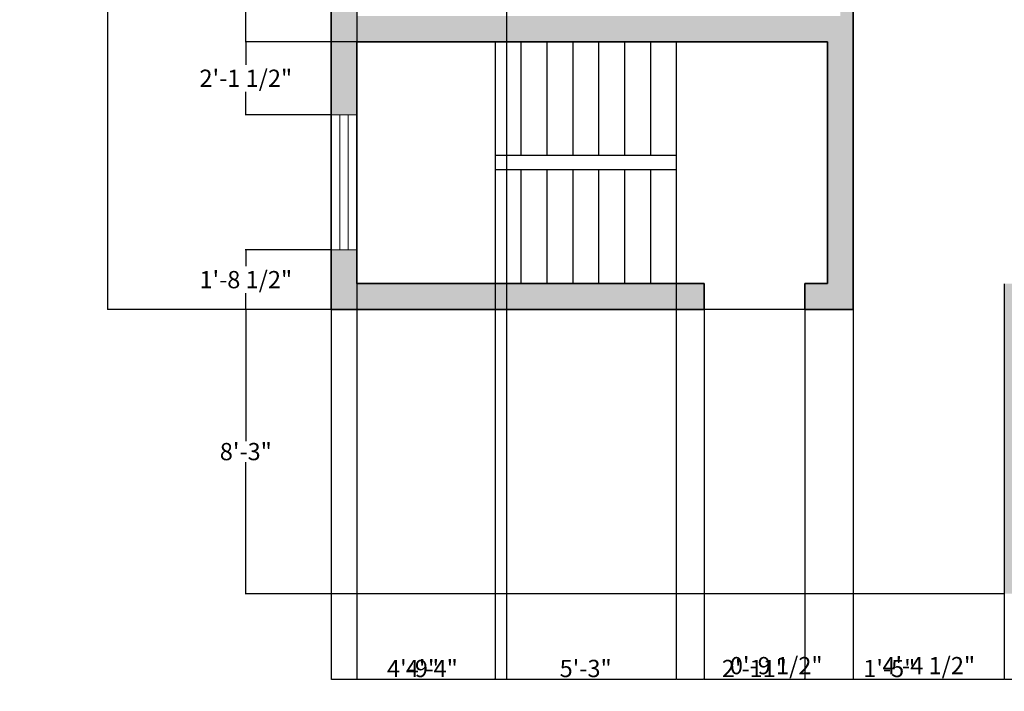
# Model space of a CAD drawing. Units: inches. Extents: x 2322 to 2932, y 142 to 762.
# Tile 1 of 7: x 2322 to 2664, y 142 to 376. Entities that reach past the tile are written whole.
import ezdxf

# ---------------------------------------------------------------- set-up
doc = ezdxf.new("R2010")
doc.units = ezdxf.units.IN
doc.header["$MEASUREMENT"] = 0
for name, color, linetype, lineweight in [('A-ANNO-DIMS', 2, 'Continuous', 18), ('A-FLOR-STRS', 7, 'Continuous', 25), ('A-GLAZ', 4, 'Continuous', 18), ('A-WALL', 7, 'Continuous', 35)]:
    doc.layers.add(name, color=color, linetype=linetype, lineweight=lineweight)
doc.layers.add('A-WALL-PATT', color=40, linetype='Continuous', lineweight=13, true_color=0xf8d731)
doc.styles.get("Standard").update_dxf_attribs({"font": 'italic8.shx'})
doc.dimstyles.get("Standard").update_dxf_attribs({"dimtxt": 6, "dimasz": 0.15, "dimexe": 0.18, "dimexo": 0.0625, "dimgap": 0.09, "dimtad": 1, "dimtih": 1, "dimtoh": 1, "dimzin": 0, "dimdsep": 46, "dimlunit": 3, "dimtxsty": 'Standard', "dimblk": 'CLOSEDBLANK', "dimcen": 0.09, "dimclrd": 3, "dimclre": 1, "dimclrt": 6, "dimadec": 0, "dimazin": 0, "dimtfac": 1, "dimtofl": 0, "dimtmove": 0, "dimatfit": 3, "dimldrblk": 'DOT', "dimfxl": 1, "dimtolj": 1, "dimtzin": 0, "dimarcsym": 0})

# ---------------------------------------------------------------- blocks, each defined once
blk = doc.blocks.new('_ClosedBlank')
at = {"color": 0, "linetype": 'ByBlock', "lineweight": -2}
for p, q in [((-1, 0.2), (0, 0)), ((-1, 0.2), (-1, -0.2)), ((0, 0), (-1, -0.2))]:
    blk.add_line(p, q, dxfattribs=at)
blk = doc.blocks.new('*D8')
at = {"layer": 'A-ANNO-DIMS', "color": 0, "lineweight": -2, "transparency": 16777216}
for p, q in [((2430, 718.82), (2352.33, 718.82)), ((2352.51, 718.67), (2352.51, 501.45)), ((2352.51, 274.91), (2352.51, 492.13)), ((2430, 274.76), (2352.33, 274.76))]:
    blk.add_line(p, q, dxfattribs=at)
at = {"layer": 'Defpoints', "color": 0, "transparency": 16777216}
for p in [(2430.06, 718.82), (2352.51, 274.76), (2430.06, 274.76)]:
    blk.add_point(p, dxfattribs=at)
at = {"layer": 'A-ANNO-DIMS', "color": 0, "lineweight": -2, "transparency": 16777216, "xscale": 0.15, "yscale": 0.15, "zscale": 0.15}
for p, rotation in [((2352.51, 718.82), 90), ((2352.51, 274.76), 270)]:
    blk.add_blockref('_ClosedBlank', p, dxfattribs=dict(at, rotation=rotation))
at = {"layer": 'A-ANNO-DIMS', "color": 0, "transparency": 16777216, "insert": (2352.51, 496.79), "char_height": 6, "attachment_point": 5}
blk.add_mtext('\\A1;37\'-0.06" [11.28]', dxfattribs=at)
blk = doc.blocks.new('_Dot')
at = {"color": 0, "linetype": 'ByBlock', "lineweight": -2}
blk.add_line((-0.5, 0), (-1, 0), dxfattribs=at)
at = {"color": 0, "linetype": 'ByBlock', "const_width": 0.5}
blk.add_lwpolyline([(-0.25, 0, 1), (0.25, 0, 1)], format="xyb", close=True, dxfattribs=at)
blk = doc.blocks.new('WINDOW-47X9')
for p, q in [((47, 9), (0, 9)), ((0, 9), (0, 0)), ((47, 0), (47, 9)), ((0, 6), (47, 6)), ((0, 3), (47, 3)), ((0, 0), (47, 0))]:
    blk.add_line(p, q)
blk = doc.blocks.new('*D44')
at = {"layer": 'A-ANNO-DIMS', "color": 1, "lineweight": -2, "transparency": 16777216}
for p, q in [((2487.06, 283.69), (2487.06, 146.01)), ((2430.06, 274.69), (2430.06, 146.01))]:
    blk.add_line(p, q, dxfattribs=at)
at = {"layer": 'A-ANNO-DIMS', "color": 3, "lineweight": -2, "transparency": 16777216}
blk.add_line((2430.21, 146.19), (2486.91, 146.19), dxfattribs=at)
at = {"layer": 'Defpoints', "color": 0, "transparency": 16777216}
for p in [(2487.06, 283.76), (2430.06, 274.76), (2487.06, 146.19)]:
    blk.add_point(p, dxfattribs=at)
at = {"layer": 'A-ANNO-DIMS', "color": 3, "lineweight": -2, "transparency": 16777216, "xscale": 0.15, "yscale": 0.15, "zscale": 0.15, "rotation": 180}
blk.add_blockref('_ClosedBlank', (2430.06, 146.19), dxfattribs=at)
at = {"layer": 'A-ANNO-DIMS', "color": 3, "lineweight": -2, "transparency": 16777216, "xscale": 0.15, "yscale": 0.15, "zscale": 0.15}
blk.add_blockref('_ClosedBlank', (2487.06, 146.19), dxfattribs=at)
at = {"layer": 'A-ANNO-DIMS', "color": 6, "transparency": 16777216, "insert": (2458.56, 149.85), "char_height": 6, "attachment_point": 5}
blk.add_mtext('\\A1;4\'-9"', dxfattribs=at)
blk = doc.blocks.new('*D45')
at = {"layer": 'A-ANNO-DIMS', "color": 1, "lineweight": -2, "transparency": 16777216}
for p, q in [((2487.06, 283.69), (2487.06, 146.01)), ((2550.06, 283.69), (2550.06, 146.01))]:
    blk.add_line(p, q, dxfattribs=at)
at = {"layer": 'A-ANNO-DIMS', "color": 3, "lineweight": -2, "transparency": 16777216}
blk.add_line((2487.21, 146.19), (2549.91, 146.19), dxfattribs=at)
at = {"layer": 'Defpoints', "color": 0, "transparency": 16777216}
for p in [(2487.06, 283.76), (2550.06, 283.76), (2550.06, 146.19)]:
    blk.add_point(p, dxfattribs=at)
at = {"layer": 'A-ANNO-DIMS', "color": 3, "lineweight": -2, "transparency": 16777216, "xscale": 0.15, "yscale": 0.15, "zscale": 0.15, "rotation": 180}
blk.add_blockref('_ClosedBlank', (2487.06, 146.19), dxfattribs=at)
at = {"layer": 'A-ANNO-DIMS', "color": 3, "lineweight": -2, "transparency": 16777216, "xscale": 0.15, "yscale": 0.15, "zscale": 0.15}
blk.add_blockref('_ClosedBlank', (2550.06, 146.19), dxfattribs=at)
at = {"layer": 'A-ANNO-DIMS', "color": 6, "transparency": 16777216, "insert": (2518.56, 149.85), "char_height": 6, "attachment_point": 5}
blk.add_mtext('\\A1;5\'-3"', dxfattribs=at)
blk = doc.blocks.new('*D46')
at = {"layer": 'A-ANNO-DIMS', "color": 1, "lineweight": -2, "transparency": 16777216}
for p, q in [((2550.06, 283.69), (2550.06, 146.01)), ((2559.69, 274.69), (2559.69, 146.01))]:
    blk.add_line(p, q, dxfattribs=at)
at = {"layer": 'A-ANNO-DIMS', "color": 3, "lineweight": -2, "transparency": 16777216}
for p, q in [((2550.21, 146.19), (2559.54, 146.19)), ((2559.69, 146.19), (2609.74, 146.19))]:
    blk.add_line(p, q, dxfattribs=at)
at = {"layer": 'Defpoints', "color": 0, "transparency": 16777216}
for p in [(2550.06, 283.76), (2559.69, 274.76), (2559.69, 146.19)]:
    blk.add_point(p, dxfattribs=at)
at = {"layer": 'A-ANNO-DIMS', "color": 3, "lineweight": -2, "transparency": 16777216, "xscale": 0.15, "yscale": 0.15, "zscale": 0.15, "rotation": 180}
blk.add_blockref('_ClosedBlank', (2550.06, 146.19), dxfattribs=at)
at = {"layer": 'A-ANNO-DIMS', "color": 3, "lineweight": -2, "transparency": 16777216, "xscale": 0.15, "yscale": 0.15, "zscale": 0.15}
blk.add_blockref('_ClosedBlank', (2559.69, 146.19), dxfattribs=at)
at = {"layer": 'A-ANNO-DIMS', "color": 6, "transparency": 16777216, "insert": (2584.79, 150.85), "char_height": 6, "attachment_point": 5}
blk.add_mtext('\\A1;0\'-9 1/2"', dxfattribs=at)
blk = doc.blocks.new('*D47')
at = {"layer": 'A-ANNO-DIMS', "color": 1, "lineweight": -2, "transparency": 16777216}
for p, q in [((2559.69, 274.69), (2559.69, 146.01)), ((2594.69, 274.69), (2594.69, 146.01))]:
    blk.add_line(p, q, dxfattribs=at)
at = {"layer": 'A-ANNO-DIMS', "color": 3, "lineweight": -2, "transparency": 16777216}
blk.add_line((2559.84, 146.19), (2594.54, 146.19), dxfattribs=at)
at = {"layer": 'Defpoints', "color": 0, "transparency": 16777216}
for p in [(2559.69, 274.76), (2594.69, 274.76), (2594.69, 146.19)]:
    blk.add_point(p, dxfattribs=at)
at = {"layer": 'A-ANNO-DIMS', "color": 3, "lineweight": -2, "transparency": 16777216, "xscale": 0.15, "yscale": 0.15, "zscale": 0.15, "rotation": 180}
blk.add_blockref('_ClosedBlank', (2559.69, 146.19), dxfattribs=at)
at = {"layer": 'A-ANNO-DIMS', "color": 3, "lineweight": -2, "transparency": 16777216, "xscale": 0.15, "yscale": 0.15, "zscale": 0.15}
blk.add_blockref('_ClosedBlank', (2594.69, 146.19), dxfattribs=at)
at = {"layer": 'A-ANNO-DIMS', "color": 6, "transparency": 16777216, "insert": (2577.19, 149.85), "char_height": 6, "attachment_point": 5}
blk.add_mtext('\\A1;2\'-11"', dxfattribs=at)
blk = doc.blocks.new('*D48')
at = {"layer": 'A-ANNO-DIMS', "color": 1, "lineweight": -2, "transparency": 16777216}
for p, q in [((2594.69, 274.69), (2594.69, 146.01)), ((2611.56, 274.69), (2611.56, 146.01))]:
    blk.add_line(p, q, dxfattribs=at)
at = {"layer": 'A-ANNO-DIMS', "color": 3, "lineweight": -2, "transparency": 16777216}
for p, q in [((2594.84, 146.19), (2611.41, 146.19)), ((2611.56, 146.19), (2636.47, 146.19))]:
    blk.add_line(p, q, dxfattribs=at)
at = {"layer": 'Defpoints', "color": 0, "transparency": 16777216}
for p in [(2594.69, 274.76), (2611.56, 274.76), (2611.56, 146.19)]:
    blk.add_point(p, dxfattribs=at)
at = {"layer": 'A-ANNO-DIMS', "color": 3, "lineweight": -2, "transparency": 16777216, "xscale": 0.15, "yscale": 0.15, "zscale": 0.15, "rotation": 180}
blk.add_blockref('_ClosedBlank', (2594.69, 146.19), dxfattribs=at)
at = {"layer": 'A-ANNO-DIMS', "color": 3, "lineweight": -2, "transparency": 16777216, "xscale": 0.15, "yscale": 0.15, "zscale": 0.15}
blk.add_blockref('_ClosedBlank', (2611.56, 146.19), dxfattribs=at)
at = {"layer": 'A-ANNO-DIMS', "color": 6, "transparency": 16777216, "insert": (2624.09, 149.85), "char_height": 6, "attachment_point": 5}
blk.add_mtext('\\A1;1\'-5"', dxfattribs=at)
blk = doc.blocks.new('*D49')
at = {"layer": 'A-ANNO-DIMS', "color": 1, "lineweight": -2, "transparency": 16777216}
for p, q in [((2664.06, 283.69), (2664.06, 146.01)), ((2611.56, 274.69), (2611.56, 146.01))]:
    blk.add_line(p, q, dxfattribs=at)
at = {"layer": 'A-ANNO-DIMS', "color": 3, "lineweight": -2, "transparency": 16777216}
blk.add_line((2611.71, 146.19), (2663.91, 146.19), dxfattribs=at)
at = {"layer": 'Defpoints', "color": 0, "transparency": 16777216}
for p in [(2664.06, 283.76), (2611.56, 274.76), (2664.06, 146.19)]:
    blk.add_point(p, dxfattribs=at)
at = {"layer": 'A-ANNO-DIMS', "color": 3, "lineweight": -2, "transparency": 16777216, "xscale": 0.15, "yscale": 0.15, "zscale": 0.15, "rotation": 180}
blk.add_blockref('_ClosedBlank', (2611.56, 146.19), dxfattribs=at)
at = {"layer": 'A-ANNO-DIMS', "color": 3, "lineweight": -2, "transparency": 16777216, "xscale": 0.15, "yscale": 0.15, "zscale": 0.15}
blk.add_blockref('_ClosedBlank', (2664.06, 146.19), dxfattribs=at)
at = {"layer": 'A-ANNO-DIMS', "color": 6, "transparency": 16777216, "insert": (2637.81, 150.85), "char_height": 6, "attachment_point": 5}
blk.add_mtext('\\A1;4\'-4 1/2"', dxfattribs=at)
blk = doc.blocks.new('*D50')
at = {"layer": 'A-ANNO-DIMS', "color": 1, "lineweight": -2, "transparency": 16777216}
for p, q in [((2611.5, 274.76), (2400.26, 274.76)), ((2664, 175.82), (2400.26, 175.82))]:
    blk.add_line(p, q, dxfattribs=at)
at = {"layer": 'A-ANNO-DIMS', "color": 3, "lineweight": -2, "transparency": 16777216}
for p, q in [((2400.44, 274.61), (2400.44, 228.95)), ((2400.44, 175.97), (2400.44, 221.63))]:
    blk.add_line(p, q, dxfattribs=at)
at = {"layer": 'Defpoints', "color": 0, "transparency": 16777216}
for p in [(2400.44, 274.76), (2611.56, 274.76), (2664.06, 175.82)]:
    blk.add_point(p, dxfattribs=at)
at = {"layer": 'A-ANNO-DIMS', "color": 3, "lineweight": -2, "transparency": 16777216, "xscale": 0.15, "yscale": 0.15, "zscale": 0.15}
for p, rotation in [((2400.44, 274.76), 90), ((2400.44, 175.82), 270)]:
    blk.add_blockref('_ClosedBlank', p, dxfattribs=dict(at, rotation=rotation))
at = {"layer": 'A-ANNO-DIMS', "color": 6, "transparency": 16777216, "insert": (2400.44, 225.29), "char_height": 6, "attachment_point": 5}
blk.add_mtext('\\A1;8\'-3"', dxfattribs=at)
blk = doc.blocks.new('*D51')
at = {"layer": 'A-ANNO-DIMS', "color": 1, "lineweight": -2, "transparency": 16777216}
for p, q in [((2439.06, 709.76), (2439.06, 146.01)), ((2491.1, 709.76), (2491.1, 146.01))]:
    blk.add_line(p, q, dxfattribs=at)
at = {"layer": 'A-ANNO-DIMS', "color": 3, "lineweight": -2, "transparency": 16777216}
blk.add_line((2439.21, 146.19), (2490.95, 146.19), dxfattribs=at)
at = {"layer": 'Defpoints', "color": 0, "transparency": 16777216}
for p in [(2439.06, 709.82), (2491.1, 709.82), (2491.1, 146.19)]:
    blk.add_point(p, dxfattribs=at)
at = {"layer": 'A-ANNO-DIMS', "color": 3, "lineweight": -2, "transparency": 16777216, "xscale": 0.15, "yscale": 0.15, "zscale": 0.15, "rotation": 180}
blk.add_blockref('_ClosedBlank', (2439.06, 146.19), dxfattribs=at)
at = {"layer": 'A-ANNO-DIMS', "color": 3, "lineweight": -2, "transparency": 16777216, "xscale": 0.15, "yscale": 0.15, "zscale": 0.15}
blk.add_blockref('_ClosedBlank', (2491.1, 146.19), dxfattribs=at)
at = {"layer": 'A-ANNO-DIMS', "color": 6, "transparency": 16777216, "insert": (2465.08, 149.85), "char_height": 6, "attachment_point": 5}
blk.add_mtext('\\A1;4\'-4"', dxfattribs=at)
blk = doc.blocks.new('*D55')
at = {"layer": 'A-ANNO-DIMS', "color": 1, "lineweight": -2, "transparency": 16777216}
for p, q in [((2430, 295.45), (2400.26, 295.45)), ((2430, 274.76), (2400.26, 274.76))]:
    blk.add_line(p, q, dxfattribs=at)
at = {"layer": 'A-ANNO-DIMS', "color": 3, "lineweight": -2, "transparency": 16777216}
for p, q in [((2400.44, 295.3), (2400.44, 289.77)), ((2400.44, 274.91), (2400.44, 280.44))]:
    blk.add_line(p, q, dxfattribs=at)
at = {"layer": 'Defpoints', "color": 0, "transparency": 16777216}
for p in [(2400.44, 295.45), (2430.06, 295.45), (2430.06, 274.76)]:
    blk.add_point(p, dxfattribs=at)
at = {"layer": 'A-ANNO-DIMS', "color": 3, "lineweight": -2, "transparency": 16777216, "xscale": 0.15, "yscale": 0.15, "zscale": 0.15}
for p, rotation in [((2400.44, 295.45), 90), ((2400.44, 274.76), 270)]:
    blk.add_blockref('_ClosedBlank', p, dxfattribs=dict(at, rotation=rotation))
at = {"layer": 'A-ANNO-DIMS', "color": 6, "transparency": 16777216, "insert": (2400.44, 285.1), "char_height": 6, "attachment_point": 5}
blk.add_mtext('\\A1;1\'-8 1/2"', dxfattribs=at)
blk = doc.blocks.new('*D56')
at = {"layer": 'A-ANNO-DIMS', "color": 1, "lineweight": -2, "transparency": 16777216}
for p, q in [((2439, 367.82), (2400.26, 367.82)), ((2430, 342.45), (2400.26, 342.45))]:
    blk.add_line(p, q, dxfattribs=at)
at = {"layer": 'A-ANNO-DIMS', "color": 3, "lineweight": -2, "transparency": 16777216}
for p, q in [((2400.44, 367.67), (2400.44, 359.8)), ((2400.44, 342.6), (2400.44, 350.47))]:
    blk.add_line(p, q, dxfattribs=at)
at = {"layer": 'Defpoints', "color": 0, "transparency": 16777216}
for p in [(2400.44, 367.82), (2439.06, 367.82), (2430.06, 342.45)]:
    blk.add_point(p, dxfattribs=at)
at = {"layer": 'A-ANNO-DIMS', "color": 3, "lineweight": -2, "transparency": 16777216, "xscale": 0.15, "yscale": 0.15, "zscale": 0.15}
for p, rotation in [((2400.44, 367.82), 90), ((2400.44, 342.45), 270)]:
    blk.add_blockref('_ClosedBlank', p, dxfattribs=dict(at, rotation=rotation))
at = {"layer": 'A-ANNO-DIMS', "color": 6, "transparency": 16777216, "insert": (2400.44, 355.14), "char_height": 6, "attachment_point": 5}
blk.add_mtext('\\A1;2\'-1 1/2"', dxfattribs=at)
blk = doc.blocks.new('*D57')
at = {"layer": 'A-ANNO-DIMS', "color": 1, "lineweight": -2, "transparency": 16777216}
for p, q in [((2430, 418.18), (2400.26, 418.18)), ((2439, 367.82), (2400.26, 367.82))]:
    blk.add_line(p, q, dxfattribs=at)
at = {"layer": 'A-ANNO-DIMS', "color": 3, "lineweight": -2, "transparency": 16777216}
for p, q in [((2400.44, 418.03), (2400.44, 397.66)), ((2400.44, 367.97), (2400.44, 388.34))]:
    blk.add_line(p, q, dxfattribs=at)
at = {"layer": 'Defpoints', "color": 0, "transparency": 16777216}
for p in [(2400.44, 418.18), (2430.06, 418.18), (2439.06, 367.82)]:
    blk.add_point(p, dxfattribs=at)
at = {"layer": 'A-ANNO-DIMS', "color": 3, "lineweight": -2, "transparency": 16777216, "xscale": 0.15, "yscale": 0.15, "zscale": 0.15}
for p, rotation in [((2400.44, 418.18), 90), ((2400.44, 367.82), 270)]:
    blk.add_blockref('_ClosedBlank', p, dxfattribs=dict(at, rotation=rotation))
at = {"layer": 'A-ANNO-DIMS', "color": 6, "transparency": 16777216, "insert": (2400.44, 393), "char_height": 6, "attachment_point": 5}
blk.add_mtext('\\A1;4\'-2 1/2"', dxfattribs=at)
blk = doc.blocks.new('*D65')
at = {"layer": 'A-ANNO-DIMS', "color": 1, "lineweight": -2, "transparency": 16777216}
for p, q in [((2664.06, 175.76), (2664.06, 146.01)), ((2710.26, 175.76), (2710.26, 146.01))]:
    blk.add_line(p, q, dxfattribs=at)
at = {"layer": 'A-ANNO-DIMS', "color": 3, "lineweight": -2, "transparency": 16777216}
blk.add_line((2664.21, 146.19), (2710.11, 146.19), dxfattribs=at)
at = {"layer": 'Defpoints', "color": 0, "transparency": 16777216}
for p in [(2664.06, 175.82), (2710.26, 175.82), (2710.26, 146.19)]:
    blk.add_point(p, dxfattribs=at)
at = {"layer": 'A-ANNO-DIMS', "color": 3, "lineweight": -2, "transparency": 16777216, "xscale": 0.15, "yscale": 0.15, "zscale": 0.15, "rotation": 180}
blk.add_blockref('_ClosedBlank', (2664.06, 146.19), dxfattribs=at)
at = {"layer": 'A-ANNO-DIMS', "color": 3, "lineweight": -2, "transparency": 16777216, "xscale": 0.15, "yscale": 0.15, "zscale": 0.15}
blk.add_blockref('_ClosedBlank', (2710.26, 146.19), dxfattribs=at)
at = {"layer": 'A-ANNO-DIMS', "color": 6, "transparency": 16777216, "insert": (2687.16, 149.85), "char_height": 6, "attachment_point": 5}
blk.add_mtext('\\A1;3\'-10"', dxfattribs=at)

msp = doc.modelspace()

# ---------------------------------------------------------------- hatches: boundary and pattern name
at = {"layer": 'A-WALL-PATT'}
h = msp.add_hatch(color=256, dxfattribs=at)
h.dxf.hatch_style = 1
h.paths.add_polyline_path([(2439.065, 709.819), (2491.097, 709.819), (2491.097, 718.819), (2430.065, 718.819), (2430.065, 663.548), (2439.065, 663.548)])
h.paths.add_polyline_path([(2704.233, 718.819), (2654.246, 718.819), (2654.246, 709.819), (2668.565, 709.819), (2668.565, 661.819), (2673.065, 661.819), (2673.065, 709.819), (2704.233, 709.819)], flags=17)
h.paths.add_polyline_path([(2624.246, 718.819), (2538.097, 718.819), (2538.097, 709.819), (2607.065, 709.819), (2607.065, 565.819), (2583.065, 565.819), (2583.065, 561.319), (2611.565, 561.319), (2611.565, 609.319), (2668.565, 609.319), (2668.565, 561.319), (2758.065, 561.319), (2758.065, 565.819), (2673.065, 565.819), (2673.065, 626.819), (2668.565, 626.819), (2668.565, 613.819), (2611.565, 613.819), (2611.565, 709.819), (2624.246, 709.819)])
h.paths.add_polyline_path([(2802.065, 718.819), (2751.233, 718.819), (2751.233, 709.819), (2793.065, 709.819), (2793.065, 660.138), (2802.065, 660.138)])
h.paths.add_polyline_path([(2802.065, 613.138), (2793.065, 613.138), (2793.065, 478.568), (2802.065, 478.568)])
h.paths.add_polyline_path([(2439.065, 616.548), (2430.065, 616.548), (2430.065, 551.562), (2439.065, 551.562), (2439.065, 561.319), (2483.455, 561.319), (2483.455, 565.819), (2439.065, 565.819)])
h.paths.add_polyline_path([(2548.065, 565.819), (2518.455, 565.819), (2518.455, 561.319), (2541.065, 561.319), (2541.065, 501.319), (2439.065, 501.319), (2439.065, 516.562), (2430.065, 516.562), (2430.065, 465.181), (2439.065, 465.181), (2439.065, 496.819), (2503.266, 496.819), (2541.065, 496.819), (2541.065, 472.819), (2545.565, 472.819), (2545.565, 561.319), (2548.065, 561.319)])
h.paths.add_polyline_path([(2439.065, 418.181), (2430.065, 418.181), (2430.065, 342.453), (2439.065, 342.453), (2439.065, 367.819), (2602.565, 367.819), (2602.565, 283.756), (2594.693, 283.756), (2594.693, 274.756), (2611.565, 274.756), (2611.565, 501.319), (2580.942, 501.319), (2580.942, 496.819), (2607.065, 496.819), (2607.065, 376.819), (2439.065, 376.819)])
h.paths.add_polyline_path([(2793.057, 530.805), (2793.057, 530.68), (2793.106, 530.68), (2793.106, 530.805)], flags=25)
h.paths.add_polyline_path([(2793.057, 530.808), (2793.057, 530.676), (2793.106, 530.676), (2793.106, 530.808)], flags=9)
h = msp.add_hatch(color=256, dxfattribs=at)
h.dxf.hatch_style = 1
h.paths.add_polyline_path([(2559.693, 283.756), (2439.065, 283.756), (2439.065, 295.453), (2430.065, 295.453), (2430.065, 274.756), (2559.693, 274.756)])
h.paths.add_polyline_path([(2802.065, 431.568), (2793.065, 431.568), (2793.065, 374.218), (2802.065, 374.218)])
h.paths.add_polyline_path([(2802.065, 327.218), (2793.065, 327.218), (2793.065, 283.756), (2708.065, 283.756), (2708.065, 279.256), (2793.065, 279.256), (2793.065, 260.879), (2802.065, 260.879)])
h.paths.add_polyline_path([(2673.065, 283.756), (2664.065, 283.756), (2664.065, 175.819), (2710.255, 175.819), (2710.255, 184.819), (2673.065, 184.819)])
h.paths.add_polyline_path([(2802.065, 213.879), (2793.065, 213.879), (2793.065, 184.819), (2757.255, 184.819), (2757.255, 175.819), (2802.065, 175.819)])

# ---------------------------------------------------------------- linework, layer by layer
at = {"layer": 'A-FLOR-STRS'}
for p, q in [((2487.065, 367.819), (2487.065, 283.756)), ((2496.065, 367.819), (2496.065, 328.219)), ((2505.065, 367.819), (2505.065, 328.219)), ((2514.065, 367.819), (2514.065, 328.219)), ((2523.065, 367.819), (2523.065, 328.219)), ((2532.065, 367.819), (2532.065, 328.219)), ((2541.065, 367.819), (2541.065, 328.219)), ((2550.065, 367.819), (2550.065, 283.756)), ((2550.065, 328.219), (2487.065, 328.219)), ((2487.065, 323.356), (2550.065, 323.356)), ((2496.065, 323.356), (2496.065, 283.756)), ((2505.065, 323.356), (2505.065, 283.756)), ((2514.065, 323.356), (2514.065, 283.756)), ((2523.065, 323.356), (2523.065, 283.756)), ((2532.065, 323.356), (2532.065, 283.756)), ((2541.065, 323.356), (2541.065, 283.756))]:
    msp.add_line(p, q, dxfattribs=at)
at = {"layer": 'A-WALL'}
for p, q in [((2430.065, 718.819), (2430.065, 274.756)), ((2611.565, 501.319), (2611.565, 274.756)), ((2602.565, 367.819), (2439.065, 367.819)), ((2439.065, 367.819), (2439.065, 283.756)), ((2602.565, 367.819), (2602.565, 283.756)), ((2439.065, 283.756), (2559.693, 283.756)), ((2559.693, 283.756), (2559.693, 274.756)), ((2594.693, 283.756), (2594.693, 274.756)), ((2594.693, 283.756), (2602.565, 283.756)), ((2430.065, 274.756), (2559.693, 274.756)), ((2594.693, 274.756), (2611.565, 274.756))]:
    msp.add_line(p, q, dxfattribs=at)

# ---------------------------------------------------------------- block references
at = {"layer": 'A-GLAZ', "rotation": 90.00000000000183}
msp.add_blockref('WINDOW-47X9', (2439.064, 295.453), dxfattribs=at)

# ---------------------------------------------------------------- dimensions: what is measured, and where the dimension line sits
at = {"layer": 'A-ANNO-DIMS'}
for base, p1, p2, override, picture, middle in [((2352.512, 274.756), (2430.065, 718.819), (2430.065, 274.756), {"dimclrd": 0, "dimclre": 0, "dimclrt": 0}, '*D8', (2352.512, 496.787)), ((2400.44, 418.181), (2439.065, 367.819), (2430.065, 418.181), {"dimdec": 1, "dimlfac": 1, "dimrnd": 0, "dimzin": 1, "dimdsep": 46, "dimlunit": 4, "dimfrac": 2}, '*D57', (2400.44, 393)), ((2400.44, 367.819), (2430.065, 342.453), (2439.065, 367.819), {"dimdec": 1, "dimlfac": 1, "dimrnd": 0, "dimzin": 1, "dimdsep": 46, "dimlunit": 4, "dimfrac": 2}, '*D56', (2400.44, 355.136)), ((2400.44, 295.453), (2430.065, 274.756), (2430.065, 295.453), {"dimdec": 1, "dimlfac": 1, "dimrnd": 0, "dimzin": 1, "dimdsep": 46, "dimlunit": 4, "dimfrac": 2}, '*D55', (2400.44, 285.105)), ((2400.44, 274.756), (2664.065, 175.819), (2611.565, 274.756), {"dimdec": 1, "dimlfac": 1, "dimrnd": 0, "dimzin": 1, "dimdsep": 46, "dimlunit": 4, "dimfrac": 2}, '*D50', (2400.44, 225.287))]:
    dim = msp.add_linear_dim(base=base, p1=p1, p2=p2, angle=90, dimstyle='Standard', override=override, dxfattribs=at)
    dim.commit()
    dim.dimension.update_dxf_attribs({"geometry": picture, "text_midpoint": middle})
for base, p1, p2, picture, middle in [((2491.097, 146.194), (2439.065, 709.819), (2491.097, 709.819), '*D51', (2465.081, 149.855)), ((2487.065, 146.194), (2430.065, 274.756), (2487.065, 283.756), '*D44', (2458.565, 149.855)), ((2550.065, 146.194), (2487.065, 283.756), (2550.065, 283.756), '*D45', (2518.565, 149.855)), ((2559.693, 146.194), (2550.065, 283.756), (2559.693, 274.756), '*D46', (2584.79, 150.855)), ((2664.065, 146.194), (2611.565, 274.756), (2664.065, 283.756), '*D49', (2637.815, 150.855)), ((2594.693, 146.194), (2559.693, 274.756), (2594.693, 274.756), '*D47', (2577.193, 149.855)), ((2611.565, 146.194), (2594.693, 274.756), (2611.565, 274.756), '*D48', (2624.09, 149.855)), ((2710.255, 146.194), (2664.065, 175.819), (2710.255, 175.819), '*D65', (2687.16, 149.855))]:
    dim = msp.add_linear_dim(base=base, p1=p1, p2=p2, dimstyle='Standard', override={"dimdec": 1, "dimlfac": 1, "dimrnd": 0, "dimzin": 1, "dimdsep": 46, "dimlunit": 4, "dimfrac": 2}, dxfattribs=at)
    dim.commit()
    dim.dimension.update_dxf_attribs({"geometry": picture, "text_midpoint": middle})

doc.saveas('drawing.dxf')
